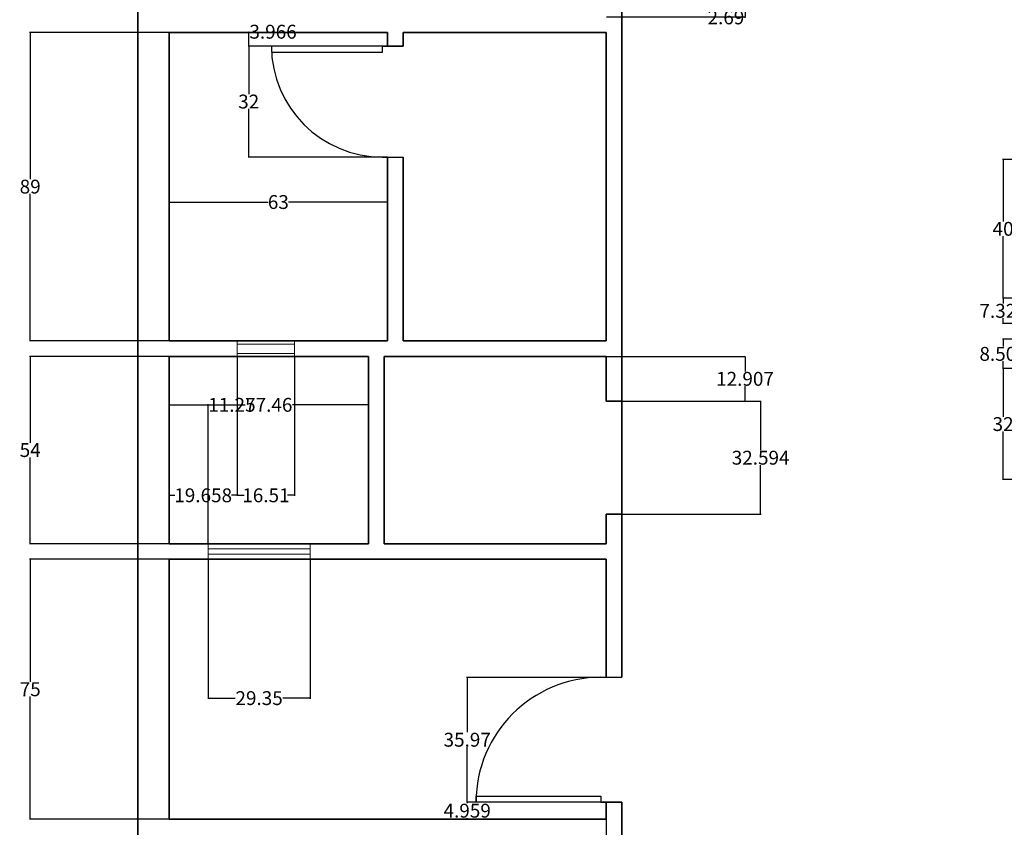
# Model space of a CAD drawing. Units: inches. Extents: x 1353 to 1853, y 16593 to 17433.
# Tile 2 of 4: x 1355 to 1639, y 16947 to 17180. Entities that reach past the tile are written whole.
import ezdxf

# ---------------------------------------------------------------- set-up
doc = ezdxf.new("R2010")
doc.units = ezdxf.units.IN
doc.header["$MEASUREMENT"] = 0
for name, color, linetype, lineweight in [('A-ANNO-DIMS', 2, 'Continuous', 18), ('A-DOOR', 3, 'Continuous', 25), ('A-GLAZ', 4, 'Continuous', 18), ('A-WALL', 7, 'Continuous', 35)]:
    doc.layers.add(name, color=color, linetype=linetype, lineweight=lineweight)
doc.styles.get("Standard").update_dxf_attribs({"font": 'arial.ttf'})
doc.dimstyles.get("Standard").update_dxf_attribs({"dimtxt": 4, "dimasz": 0.18, "dimexe": 0.18, "dimexo": 0.0625, "dimgap": 0.09, "dimtad": 0, "dimtih": 1, "dimtoh": 1, "dimdec": 0, "dimzin": 0, "dimdsep": 46, "dimlunit": 3, "dimtxsty": 'Standard', "dimcen": 0.09, "dimadec": 0, "dimazin": 0, "dimtfac": 1, "dimtdec": 0, "dimtofl": 0, "dimtmove": 0, "dimatfit": 3, "dimfxl": 1, "dimtolj": 1, "dimtzin": 0, "dimarcsym": 0})

# ---------------------------------------------------------------- blocks, each defined once
blk = doc.blocks.new('*U3')
for p, q in [((0, 0), (0, -6)), ((36, 0), (36, -6))]:
    blk.add_line(p, q)
blk.add_lwpolyline([(0, 0), (0, 36), (1.75, 36), (1.75, 0)], close=True)
blk.add_arc((0, 0), 36, 0, 90)
blk = doc.blocks.new('*U8')
for p, q in [((0, 0), (0, -6)), ((-32, 0), (-32, -6))]:
    blk.add_line(p, q)
blk.add_lwpolyline([(0, 0), (0, 32), (-1.75, 32), (-1.75, 0)], close=True)
blk.add_arc((0, 0), 32, 90, 180)
blk = doc.blocks.new('*D17')
at = {"layer": 'A-ANNO-DIMS', "color": 0, "lineweight": -2, "transparency": 16777216}
for p, q in [((1397.82, 17176.28), (1357.65, 17176.28)), ((1357.83, 17176.1), (1357.83, 17133.91)), ((1357.83, 17087.46), (1357.83, 17129.65)), ((1397.82, 17087.28), (1357.65, 17087.28))]:
    blk.add_line(p, q, dxfattribs=at)
at = {"layer": 'A-ANNO-DIMS', "color": 0, "transparency": 16777216}
for points in [[(1357.8, 17176.1), (1357.86, 17176.1), (1357.83, 17176.28)], [(1357.8, 17087.46), (1357.86, 17087.46), (1357.83, 17087.28)]]:
    blk.add_solid(points, dxfattribs=at)
at = {"layer": 'Defpoints', "color": 0, "transparency": 16777216}
for p in [(1357.83, 17176.28), (1397.88, 17176.28), (1397.88, 17087.28)]:
    blk.add_point(p, dxfattribs=at)
at = {"layer": 'A-ANNO-DIMS', "color": 0, "transparency": 16777216, "insert": (1357.83, 17131.78), "char_height": 4, "attachment_point": 5}
blk.add_mtext('\\A1;89', dxfattribs=at)
blk = doc.blocks.new('*D18')
at = {"layer": 'A-ANNO-DIMS', "color": 0, "lineweight": -2, "transparency": 16777216}
for p, q in [((1397.82, 17082.78), (1357.65, 17082.78)), ((1357.83, 17082.6), (1357.83, 17057.9)), ((1357.83, 17028.96), (1357.83, 17053.66)), ((1397.82, 17028.78), (1357.65, 17028.78))]:
    blk.add_line(p, q, dxfattribs=at)
at = {"layer": 'A-ANNO-DIMS', "color": 0, "transparency": 16777216}
for points in [[(1357.8, 17082.6), (1357.86, 17082.6), (1357.83, 17082.78)], [(1357.8, 17028.96), (1357.86, 17028.96), (1357.83, 17028.78)]]:
    blk.add_solid(points, dxfattribs=at)
at = {"layer": 'Defpoints', "color": 0, "transparency": 16777216}
for p in [(1357.83, 17082.78), (1397.88, 17082.78), (1397.88, 17028.78)]:
    blk.add_point(p, dxfattribs=at)
at = {"layer": 'A-ANNO-DIMS', "color": 0, "transparency": 16777216, "insert": (1357.83, 17055.78), "char_height": 4, "attachment_point": 5}
blk.add_mtext('\\A1;54', dxfattribs=at)
blk = doc.blocks.new('*D19')
at = {"layer": 'A-ANNO-DIMS', "color": 0, "lineweight": -2, "transparency": 16777216}
for p, q in [((1397.82, 17024.28), (1357.65, 17024.28)), ((1357.83, 17024.1), (1357.83, 16988.9)), ((1357.83, 16949.46), (1357.83, 16984.66)), ((1397.82, 16949.28), (1357.65, 16949.28))]:
    blk.add_line(p, q, dxfattribs=at)
at = {"layer": 'A-ANNO-DIMS', "color": 0, "transparency": 16777216}
for points in [[(1357.8, 17024.1), (1357.86, 17024.1), (1357.83, 17024.28)], [(1357.8, 16949.46), (1357.86, 16949.46), (1357.83, 16949.28)]]:
    blk.add_solid(points, dxfattribs=at)
at = {"layer": 'Defpoints', "color": 0, "transparency": 16777216}
for p in [(1357.83, 17024.28), (1397.88, 17024.28), (1397.88, 16949.28)]:
    blk.add_point(p, dxfattribs=at)
at = {"layer": 'A-ANNO-DIMS', "color": 0, "transparency": 16777216, "insert": (1357.83, 16986.78), "char_height": 4, "attachment_point": 5}
blk.add_mtext('\\A1;75', dxfattribs=at)
blk = doc.blocks.new('*D30')
at = {"layer": 'A-ANNO-DIMS', "color": 0, "lineweight": -2, "transparency": 16777216}
for p, q in [((1397.88, 17087.34), (1397.88, 17127.51)), ((1398.06, 17127.33), (1426.42, 17127.33)), ((1460.7, 17127.33), (1432.35, 17127.33)), ((1460.88, 17087.34), (1460.88, 17127.51))]:
    blk.add_line(p, q, dxfattribs=at)
at = {"layer": 'A-ANNO-DIMS', "color": 0, "transparency": 16777216}
for points in [[(1398.06, 17127.36), (1398.06, 17127.3), (1397.88, 17127.33)], [(1460.7, 17127.36), (1460.7, 17127.3), (1460.88, 17127.33)]]:
    blk.add_solid(points, dxfattribs=at)
at = {"layer": 'Defpoints', "color": 0, "transparency": 16777216}
for p in [(1460.88, 17127.33), (1397.88, 17087.28), (1460.88, 17087.28)]:
    blk.add_point(p, dxfattribs=at)
at = {"layer": 'A-ANNO-DIMS', "color": 0, "transparency": 16777216, "insert": (1429.38, 17127.33), "char_height": 4, "attachment_point": 5}
blk.add_mtext('\\A1;63', dxfattribs=at)
blk = doc.blocks.new('*D31')
at = {"layer": 'A-ANNO-DIMS', "color": 0, "lineweight": -2, "transparency": 16777216}
for p, q in [((1397.88, 17028.84), (1397.88, 17069.01)), ((1398.06, 17068.83), (1419.78, 17068.83)), ((1455.17, 17068.83), (1433.45, 17068.83)), ((1455.35, 17028.84), (1455.35, 17069.01))]:
    blk.add_line(p, q, dxfattribs=at)
at = {"layer": 'A-ANNO-DIMS', "color": 0, "transparency": 16777216}
for points in [[(1398.06, 17068.86), (1398.06, 17068.8), (1397.88, 17068.83)], [(1455.17, 17068.86), (1455.17, 17068.8), (1455.35, 17068.83)]]:
    blk.add_solid(points, dxfattribs=at)
at = {"layer": 'Defpoints', "color": 0, "transparency": 16777216}
for p in [(1455.35, 17068.83), (1397.88, 17028.78), (1455.35, 17028.78)]:
    blk.add_point(p, dxfattribs=at)
at = {"layer": 'A-ANNO-DIMS', "color": 0, "transparency": 16777216, "insert": (1426.62, 17068.83), "char_height": 4, "attachment_point": 5}
blk.add_mtext('\\A1;57.46', dxfattribs=at)
blk = doc.blocks.new('*D33')
at = {"layer": 'A-ANNO-DIMS', "color": 0, "lineweight": -2, "transparency": 16777216}
for p, q in [((1523.88, 16954.18), (1523.88, 16914.01)), ((1528.38, 16954.18), (1528.38, 16914.01)), ((1523.88, 16914.19), (1523.7, 16914.19)), ((1528.2, 16914.19), (1524.06, 16914.19))]:
    blk.add_line(p, q, dxfattribs=at)
at = {"layer": 'A-ANNO-DIMS', "color": 0, "transparency": 16777216}
for points in [[(1524.06, 16914.22), (1524.06, 16914.16), (1523.88, 16914.19)], [(1528.2, 16914.22), (1528.2, 16914.16), (1528.38, 16914.19)]]:
    blk.add_solid(points, dxfattribs=at)
at = {"layer": 'Defpoints', "color": 0, "transparency": 16777216}
for p in [(1523.88, 16954.24), (1528.38, 16954.24), (1523.88, 16914.19)]:
    blk.add_point(p, dxfattribs=at)
at = {"layer": 'A-ANNO-DIMS', "color": 0, "transparency": 16777216, "insert": (1519.88, 16914.19), "char_height": 4, "attachment_point": 5}
blk.add_mtext('\\A1;4.5', dxfattribs=at)
blk = doc.blocks.new('*D56')
at = {"layer": 'A-ANNO-DIMS', "color": 0, "lineweight": -2, "transparency": 16777216}
for p, q in [((1523.95, 17183.47), (1564.11, 17183.47)), ((1563.93, 17183.29), (1563.93, 17180.96)), ((1523.95, 17180.78), (1564.11, 17180.78)), ((1563.93, 17180.6), (1563.75, 17180.6)), ((1563.93, 17180.78), (1563.93, 17180.6))]:
    blk.add_line(p, q, dxfattribs=at)
at = {"layer": 'A-ANNO-DIMS', "color": 0, "transparency": 16777216}
for points in [[(1563.9, 17183.29), (1563.96, 17183.29), (1563.93, 17183.47)], [(1563.9, 17180.96), (1563.96, 17180.96), (1563.93, 17180.78)]]:
    blk.add_solid(points, dxfattribs=at)
at = {"layer": 'Defpoints', "color": 0, "transparency": 16777216}
for p in [(1523.88, 17183.47), (1523.88, 17180.78), (1563.93, 17180.78)]:
    blk.add_point(p, dxfattribs=at)
at = {"layer": 'A-ANNO-DIMS', "color": 0, "transparency": 16777216, "insert": (1558.43, 17180.6), "char_height": 4, "attachment_point": 5}
blk.add_mtext('\\A1;2.69', dxfattribs=at)
blk = doc.blocks.new('*D57')
at = {"layer": 'A-ANNO-DIMS', "color": 0, "lineweight": -2, "transparency": 16777216}
for p, q in [((1460.82, 17172.32), (1420.65, 17172.32)), ((1420.83, 17172.14), (1420.83, 17158.45)), ((1420.83, 17140.5), (1420.83, 17154.18)), ((1460.82, 17140.32), (1420.65, 17140.32))]:
    blk.add_line(p, q, dxfattribs=at)
at = {"layer": 'A-ANNO-DIMS', "color": 0, "transparency": 16777216}
for points in [[(1420.8, 17172.14), (1420.86, 17172.14), (1420.83, 17172.32)], [(1420.8, 17140.5), (1420.86, 17140.5), (1420.83, 17140.32)]]:
    blk.add_solid(points, dxfattribs=at)
at = {"layer": 'Defpoints', "color": 0, "transparency": 16777216}
for p in [(1420.83, 17172.32), (1460.88, 17172.32), (1460.88, 17140.32)]:
    blk.add_point(p, dxfattribs=at)
at = {"layer": 'A-ANNO-DIMS', "color": 0, "transparency": 16777216, "insert": (1420.83, 17156.32), "char_height": 4, "attachment_point": 5}
blk.add_mtext('\\A1;32', dxfattribs=at)
blk = doc.blocks.new('*D58')
at = {"layer": 'A-ANNO-DIMS', "color": 0, "lineweight": -2, "transparency": 16777216}
for p, q in [((1460.82, 17176.28), (1420.65, 17176.28)), ((1420.83, 17176.28), (1420.83, 17176.46)), ((1420.83, 17176.46), (1421.01, 17176.46)), ((1420.83, 17172.5), (1420.83, 17176.1)), ((1460.82, 17172.32), (1420.65, 17172.32))]:
    blk.add_line(p, q, dxfattribs=at)
at = {"layer": 'A-ANNO-DIMS', "color": 0, "transparency": 16777216}
for points in [[(1420.8, 17176.1), (1420.86, 17176.1), (1420.83, 17176.28)], [(1420.8, 17172.5), (1420.86, 17172.5), (1420.83, 17172.32)]]:
    blk.add_solid(points, dxfattribs=at)
at = {"layer": 'Defpoints', "color": 0, "transparency": 16777216}
for p in [(1420.83, 17176.28), (1460.88, 17176.28), (1460.88, 17172.32)]:
    blk.add_point(p, dxfattribs=at)
at = {"layer": 'A-ANNO-DIMS', "color": 0, "transparency": 16777216, "insert": (1427.85, 17176.46), "char_height": 4, "attachment_point": 5}
blk.add_mtext('\\A1;3.966', dxfattribs=at)
blk = doc.blocks.new('*D59')
at = {"layer": 'A-ANNO-DIMS', "color": 0, "lineweight": -2, "transparency": 16777216}
for p, q in [((1523.82, 16990.21), (1483.65, 16990.21)), ((1483.83, 16990.03), (1483.83, 16974.36)), ((1483.83, 16954.42), (1483.83, 16970.09)), ((1523.82, 16954.24), (1483.65, 16954.24))]:
    blk.add_line(p, q, dxfattribs=at)
at = {"layer": 'A-ANNO-DIMS', "color": 0, "transparency": 16777216}
for points in [[(1483.8, 16990.03), (1483.86, 16990.03), (1483.83, 16990.21)], [(1483.8, 16954.42), (1483.86, 16954.42), (1483.83, 16954.24)]]:
    blk.add_solid(points, dxfattribs=at)
at = {"layer": 'Defpoints', "color": 0, "transparency": 16777216}
for p in [(1483.83, 16990.21), (1523.88, 16990.21), (1523.88, 16954.24)]:
    blk.add_point(p, dxfattribs=at)
at = {"layer": 'A-ANNO-DIMS', "color": 0, "transparency": 16777216, "insert": (1483.83, 16972.22), "char_height": 4, "attachment_point": 5}
blk.add_mtext('\\A1;35.97', dxfattribs=at)
blk = doc.blocks.new('*D61')
at = {"layer": 'A-ANNO-DIMS', "color": 0, "lineweight": -2, "transparency": 16777216}
for p, q in [((1678.32, 17139.6), (1638.15, 17139.6)), ((1638.33, 17139.42), (1638.33, 17121.73)), ((1638.33, 17099.78), (1638.33, 17117.47)), ((1678.32, 17099.6), (1638.15, 17099.6))]:
    blk.add_line(p, q, dxfattribs=at)
at = {"layer": 'A-ANNO-DIMS', "color": 0, "transparency": 16777216}
for points in [[(1638.3, 17139.42), (1638.36, 17139.42), (1638.33, 17139.6)], [(1638.3, 17099.78), (1638.36, 17099.78), (1638.33, 17099.6)]]:
    blk.add_solid(points, dxfattribs=at)
at = {"layer": 'Defpoints', "color": 0, "transparency": 16777216}
for p in [(1638.33, 17139.6), (1678.38, 17139.6), (1678.38, 17099.6)]:
    blk.add_point(p, dxfattribs=at)
at = {"layer": 'A-ANNO-DIMS', "color": 0, "transparency": 16777216, "insert": (1638.33, 17119.6), "char_height": 4, "attachment_point": 5}
blk.add_mtext('\\A1;40', dxfattribs=at)
blk = doc.blocks.new('*D62')
at = {"layer": 'A-ANNO-DIMS', "color": 0, "lineweight": -2, "transparency": 16777216}
for p, q in [((1678.32, 17079.28), (1638.15, 17079.28)), ((1638.33, 17079.1), (1638.33, 17065.41)), ((1638.33, 17047.46), (1638.33, 17061.14)), ((1678.32, 17047.28), (1638.15, 17047.28))]:
    blk.add_line(p, q, dxfattribs=at)
at = {"layer": 'A-ANNO-DIMS', "color": 0, "transparency": 16777216}
for points in [[(1638.3, 17079.1), (1638.36, 17079.1), (1638.33, 17079.28)], [(1638.3, 17047.46), (1638.36, 17047.46), (1638.33, 17047.28)]]:
    blk.add_solid(points, dxfattribs=at)
at = {"layer": 'Defpoints', "color": 0, "transparency": 16777216}
for p in [(1638.33, 17079.28), (1678.38, 17079.28), (1678.38, 17047.28)]:
    blk.add_point(p, dxfattribs=at)
at = {"layer": 'A-ANNO-DIMS', "color": 0, "transparency": 16777216, "insert": (1638.33, 17063.28), "char_height": 4, "attachment_point": 5}
blk.add_mtext('\\A1;32', dxfattribs=at)
blk = doc.blocks.new('*D68')
at = {"layer": 'A-ANNO-DIMS', "color": 0, "lineweight": -2, "transparency": 16777216}
for p, q in [((1397.88, 17082.72), (1397.88, 17042.55)), ((1417.54, 17082.72), (1417.54, 17042.55)), ((1398.06, 17042.73), (1399.5, 17042.73)), ((1417.36, 17042.73), (1415.92, 17042.73))]:
    blk.add_line(p, q, dxfattribs=at)
at = {"layer": 'A-ANNO-DIMS', "color": 0, "transparency": 16777216}
for points in [[(1398.06, 17042.76), (1398.06, 17042.7), (1397.88, 17042.73)], [(1417.36, 17042.76), (1417.36, 17042.7), (1417.54, 17042.73)]]:
    blk.add_solid(points, dxfattribs=at)
at = {"layer": 'Defpoints', "color": 0, "transparency": 16777216}
for p in [(1397.88, 17082.78), (1417.54, 17082.78), (1397.88, 17042.73)]:
    blk.add_point(p, dxfattribs=at)
at = {"layer": 'A-ANNO-DIMS', "color": 0, "transparency": 16777216, "insert": (1407.71, 17042.73), "char_height": 4, "attachment_point": 5}
blk.add_mtext('\\A1;19.658', dxfattribs=at)
blk = doc.blocks.new('*D69')
at = {"layer": 'A-ANNO-DIMS', "color": 0, "lineweight": -2, "transparency": 16777216}
for p, q in [((1417.54, 17082.72), (1417.54, 17042.55)), ((1434.05, 17082.72), (1434.05, 17042.55)), ((1417.72, 17042.73), (1419.53, 17042.73)), ((1433.87, 17042.73), (1432.06, 17042.73))]:
    blk.add_line(p, q, dxfattribs=at)
at = {"layer": 'A-ANNO-DIMS', "color": 0, "transparency": 16777216}
for points in [[(1417.72, 17042.76), (1417.72, 17042.7), (1417.54, 17042.73)], [(1433.87, 17042.76), (1433.87, 17042.7), (1434.05, 17042.73)]]:
    blk.add_solid(points, dxfattribs=at)
at = {"layer": 'Defpoints', "color": 0, "transparency": 16777216}
for p in [(1417.54, 17082.78), (1434.05, 17082.78), (1417.54, 17042.73)]:
    blk.add_point(p, dxfattribs=at)
at = {"layer": 'A-ANNO-DIMS', "color": 0, "transparency": 16777216, "insert": (1425.8, 17042.73), "char_height": 4, "attachment_point": 5}
blk.add_mtext('\\A1;16.51', dxfattribs=at)
blk = doc.blocks.new('*D70')
at = {"layer": 'A-ANNO-DIMS', "color": 0, "lineweight": -2, "transparency": 16777216}
for p, q in [((1397.88, 17028.84), (1397.88, 17069.01)), ((1398.06, 17068.83), (1408.97, 17068.83)), ((1409.15, 17028.84), (1409.15, 17069.01)), ((1409.15, 17068.83), (1409.33, 17068.83))]:
    blk.add_line(p, q, dxfattribs=at)
at = {"layer": 'A-ANNO-DIMS', "color": 0, "transparency": 16777216}
for points in [[(1398.06, 17068.86), (1398.06, 17068.8), (1397.88, 17068.83)], [(1408.97, 17068.86), (1408.97, 17068.8), (1409.15, 17068.83)]]:
    blk.add_solid(points, dxfattribs=at)
at = {"layer": 'Defpoints', "color": 0, "transparency": 16777216}
for p in [(1409.15, 17068.83), (1397.88, 17028.78), (1409.15, 17028.78)]:
    blk.add_point(p, dxfattribs=at)
at = {"layer": 'A-ANNO-DIMS', "color": 0, "transparency": 16777216, "insert": (1415.99, 17068.83), "char_height": 4, "attachment_point": 5}
blk.add_mtext('\\A1;11.27', dxfattribs=at)
blk = doc.blocks.new('*D71')
at = {"layer": 'A-ANNO-DIMS', "color": 0, "lineweight": -2, "transparency": 16777216}
for p, q in [((1409.15, 17024.22), (1409.15, 16984.05)), ((1438.51, 17024.22), (1438.51, 16984.05)), ((1409.33, 16984.23), (1416.94, 16984.23)), ((1438.33, 16984.23), (1430.72, 16984.23))]:
    blk.add_line(p, q, dxfattribs=at)
at = {"layer": 'A-ANNO-DIMS', "color": 0, "transparency": 16777216}
for points in [[(1409.33, 16984.26), (1409.33, 16984.2), (1409.15, 16984.23)], [(1438.33, 16984.26), (1438.33, 16984.2), (1438.51, 16984.23)]]:
    blk.add_solid(points, dxfattribs=at)
at = {"layer": 'Defpoints', "color": 0, "transparency": 16777216}
for p in [(1409.15, 17024.28), (1438.51, 17024.28), (1409.15, 16984.23)]:
    blk.add_point(p, dxfattribs=at)
at = {"layer": 'A-ANNO-DIMS', "color": 0, "transparency": 16777216, "insert": (1423.83, 16984.23), "char_height": 4, "attachment_point": 5}
blk.add_mtext('\\A1;29.35', dxfattribs=at)
blk = doc.blocks.new('*D72')
at = {"layer": 'A-ANNO-DIMS', "color": 0, "lineweight": -2, "transparency": 16777216}
for p, q in [((1528.45, 17069.87), (1568.61, 17069.87)), ((1568.43, 17069.69), (1568.43, 17055.71)), ((1568.43, 17037.46), (1568.43, 17051.44)), ((1528.45, 17037.28), (1568.61, 17037.28))]:
    blk.add_line(p, q, dxfattribs=at)
at = {"layer": 'A-ANNO-DIMS', "color": 0, "transparency": 16777216}
for points in [[(1568.4, 17069.69), (1568.46, 17069.69), (1568.43, 17069.87)], [(1568.4, 17037.46), (1568.46, 17037.46), (1568.43, 17037.28)]]:
    blk.add_solid(points, dxfattribs=at)
at = {"layer": 'Defpoints', "color": 0, "transparency": 16777216}
for p in [(1528.38, 17069.87), (1528.38, 17037.28), (1568.43, 17037.28)]:
    blk.add_point(p, dxfattribs=at)
at = {"layer": 'A-ANNO-DIMS', "color": 0, "transparency": 16777216, "insert": (1568.43, 17053.58), "char_height": 4, "attachment_point": 5}
blk.add_mtext('\\A1;32.594', dxfattribs=at)
blk = doc.blocks.new('*D73')
at = {"layer": 'A-ANNO-DIMS', "color": 0, "lineweight": -2, "transparency": 16777216}
for p, q in [((1523.95, 17082.78), (1564.11, 17082.78)), ((1563.93, 17082.6), (1563.93, 17078.46)), ((1563.93, 17070.05), (1563.93, 17074.2)), ((1523.95, 17069.87), (1564.11, 17069.87))]:
    blk.add_line(p, q, dxfattribs=at)
at = {"layer": 'A-ANNO-DIMS', "color": 0, "transparency": 16777216}
for points in [[(1563.9, 17082.6), (1563.96, 17082.6), (1563.93, 17082.78)], [(1563.9, 17070.05), (1563.96, 17070.05), (1563.93, 17069.87)]]:
    blk.add_solid(points, dxfattribs=at)
at = {"layer": 'Defpoints', "color": 0, "transparency": 16777216}
for p in [(1523.88, 17082.78), (1523.88, 17069.87), (1563.93, 17069.87)]:
    blk.add_point(p, dxfattribs=at)
at = {"layer": 'A-ANNO-DIMS', "color": 0, "transparency": 16777216, "insert": (1563.93, 17076.33), "char_height": 4, "attachment_point": 5}
blk.add_mtext('\\A1;12.907', dxfattribs=at)
blk = doc.blocks.new('*D74')
at = {"layer": 'A-ANNO-DIMS', "color": 0, "lineweight": -2, "transparency": 16777216}
for p, q in [((1678.32, 17087.78), (1638.15, 17087.78)), ((1638.33, 17087.6), (1638.33, 17085.66)), ((1638.33, 17079.46), (1638.33, 17081.4)), ((1678.32, 17079.28), (1638.15, 17079.28))]:
    blk.add_line(p, q, dxfattribs=at)
at = {"layer": 'A-ANNO-DIMS', "color": 0, "transparency": 16777216}
for points in [[(1638.3, 17087.6), (1638.36, 17087.6), (1638.33, 17087.78)], [(1638.3, 17079.46), (1638.36, 17079.46), (1638.33, 17079.28)]]:
    blk.add_solid(points, dxfattribs=at)
at = {"layer": 'Defpoints', "color": 0, "transparency": 16777216}
for p in [(1638.33, 17087.78), (1678.38, 17087.78), (1678.38, 17079.28)]:
    blk.add_point(p, dxfattribs=at)
at = {"layer": 'A-ANNO-DIMS', "color": 0, "transparency": 16777216, "insert": (1638.33, 17083.53), "char_height": 4, "attachment_point": 5}
blk.add_mtext('\\A1;8.504', dxfattribs=at)
blk = doc.blocks.new('*D75')
at = {"layer": 'A-ANNO-DIMS', "color": 0, "lineweight": -2, "transparency": 16777216}
for p, q in [((1678.32, 17099.6), (1638.15, 17099.6)), ((1638.33, 17099.42), (1638.33, 17098.08)), ((1638.33, 17092.46), (1638.33, 17093.81)), ((1678.32, 17092.28), (1638.15, 17092.28))]:
    blk.add_line(p, q, dxfattribs=at)
at = {"layer": 'A-ANNO-DIMS', "color": 0, "transparency": 16777216}
for points in [[(1638.3, 17099.42), (1638.36, 17099.42), (1638.33, 17099.6)], [(1638.3, 17092.46), (1638.36, 17092.46), (1638.33, 17092.28)]]:
    blk.add_solid(points, dxfattribs=at)
at = {"layer": 'Defpoints', "color": 0, "transparency": 16777216}
for p in [(1638.33, 17099.6), (1678.38, 17099.6), (1678.38, 17092.28)]:
    blk.add_point(p, dxfattribs=at)
at = {"layer": 'A-ANNO-DIMS', "color": 0, "transparency": 16777216, "insert": (1638.33, 17095.94), "char_height": 4, "attachment_point": 5}
blk.add_mtext('\\A1;7.321', dxfattribs=at)
blk = doc.blocks.new('*D76')
at = {"layer": 'A-ANNO-DIMS', "color": 0, "lineweight": -2, "transparency": 16777216}
for p, q in [((1523.82, 16954.24), (1483.65, 16954.24)), ((1483.83, 16954.06), (1483.83, 16953.89)), ((1523.82, 16949.28), (1483.65, 16949.28)), ((1483.83, 16949.46), (1483.83, 16949.63))]:
    blk.add_line(p, q, dxfattribs=at)
at = {"layer": 'A-ANNO-DIMS', "color": 0, "transparency": 16777216}
for points in [[(1483.8, 16954.06), (1483.86, 16954.06), (1483.83, 16954.24)], [(1483.8, 16949.46), (1483.86, 16949.46), (1483.83, 16949.28)]]:
    blk.add_solid(points, dxfattribs=at)
at = {"layer": 'Defpoints', "color": 0, "transparency": 16777216}
for p in [(1483.83, 16954.24), (1523.88, 16954.24), (1523.88, 16949.28)]:
    blk.add_point(p, dxfattribs=at)
at = {"layer": 'A-ANNO-DIMS', "color": 0, "transparency": 16777216, "insert": (1483.83, 16951.76), "char_height": 4, "attachment_point": 5}
blk.add_mtext('\\A1;4.959', dxfattribs=at)

msp = doc.modelspace()

# ---------------------------------------------------------------- linework, layer by layer
at = {"layer": 'A-GLAZ'}
for p, q in [((1417.5423, 17082.7809), (1417.5423, 17087.2809)), ((1417.5423, 17087.2809), (1434.0526, 17087.2809)), ((1434.0526, 17087.2809), (1434.0526, 17082.7809)), ((1434.0526, 17086.3524), (1417.5423, 17086.3524)), ((1417.5423, 17082.7809), (1417.5423, 17084.555)), ((1417.5423, 17084.555), (1417.5423, 17083.6679)), ((1434.0526, 17083.6679), (1434.0526, 17086.3524)), ((1417.5423, 17083.6679), (1434.0526, 17083.6679)), ((1434.0526, 17082.7809), (1417.5423, 17082.7809)), ((1417.5423, 17082.7809), (1417.5423, 17082.7809)), ((1409.1544, 17024.2809), (1409.1544, 17028.7809)), ((1409.1544, 17028.7809), (1438.5066, 17028.7809)), ((1438.5066, 17027.2646), (1409.1544, 17027.2646)), ((1438.5066, 17028.7809), (1438.5066, 17024.2809)), ((1438.5066, 17025.1249), (1438.5066, 17027.2646)), ((1438.5066, 17025.7421), (1409.1544, 17025.7421)), ((1409.1544, 17024.2809), (1409.1544, 17025.1249)), ((1438.5066, 17024.2809), (1409.1544, 17024.2809)), ((1409.1544, 17024.2809), (1409.1544, 17024.2809)), ((1438.5066, 17025.1249), (1438.5066, 17025.7421))]:
    msp.add_line(p, q, dxfattribs=at)
at = {"layer": 'A-WALL'}
for p, q in [((1388.8844, 16635.7809), (1388.8844, 17432.7809)), ((1528.3844, 17176.2809), (1528.3844, 17183.4674)), ((1397.8844, 17176.2809), (1455.9979, 17176.2809)), ((1397.8844, 17087.2809), (1397.8844, 17176.2809)), ((1455.9979, 17176.2809), (1460.8844, 17176.2809)), ((1460.8844, 17172.3152), (1460.8844, 17176.2809)), ((1465.3844, 17176.2809), (1523.8844, 17176.2809)), ((1465.3844, 17172.3152), (1465.3844, 17176.2809)), ((1523.8844, 17176.2809), (1523.8844, 17168.5457)), ((1528.3844, 17176.2809), (1528.3844, 17168.5457)), ((1465.3844, 17172.3152), (1460.8844, 17172.3152)), ((1523.8844, 17133.8664), (1523.8844, 17168.5457)), ((1528.3844, 17133.8664), (1528.3844, 17168.5457)), ((1460.8844, 17087.2809), (1460.8844, 17140.3152)), ((1465.3844, 17087.2809), (1465.3844, 17140.3152)), ((1523.8844, 17133.8664), (1523.8844, 17087.2809)), ((1528.3844, 17133.8664), (1528.3844, 17082.7809)), ((1397.8844, 17087.2809), (1460.8844, 17087.2809)), ((1465.3844, 17087.2809), (1523.8844, 17087.2809)), ((1397.8844, 17082.7809), (1445.8844, 17082.7809)), ((1397.8844, 17028.7809), (1397.8844, 17082.7809)), ((1445.8844, 17082.7809), (1455.3459, 17082.7809)), ((1455.3459, 17028.7809), (1455.3459, 17082.7809)), ((1459.8459, 17028.7809), (1459.8459, 17082.7809)), ((1459.8459, 17082.7809), (1465.3844, 17082.7809)), ((1465.3844, 17082.7809), (1523.8844, 17082.7809)), ((1523.8844, 17082.7809), (1523.8844, 17069.8743)), ((1528.3844, 17082.7809), (1528.3844, 17069.8743)), ((1528.3844, 17069.8743), (1523.8844, 17069.8743)), ((1528.3844, 17037.2799), (1528.3844, 17069.8743)), ((1523.8844, 17037.2799), (1528.3844, 17037.2799)), ((1523.8844, 17037.2799), (1523.8844, 17028.7809)), ((1528.3844, 17037.2799), (1528.3844, 17024.2809)), ((1397.8844, 17028.7809), (1445.8844, 17028.7809)), ((1445.8844, 17028.7809), (1455.3459, 17028.7809)), ((1459.8459, 17028.7809), (1523.8844, 17028.7809)), ((1397.8844, 17024.2809), (1450.3844, 17024.2809)), ((1397.8844, 16949.2809), (1397.8844, 17024.2809)), ((1450.3844, 17024.2809), (1459.8459, 17024.2809)), ((1459.8459, 17024.2809), (1523.8844, 17024.2809)), ((1523.8844, 17024.2809), (1523.8844, 16990.2086)), ((1528.3844, 17024.2809), (1528.3844, 16990.2398)), ((1523.8844, 16949.2809), (1523.8844, 16954.2398)), ((1523.8844, 16954.2398), (1528.3844, 16954.2398)), ((1528.3844, 16944.7809), (1528.3844, 16954.2398)), ((1397.8844, 16949.2809), (1459.8459, 16949.2809)), ((1459.8459, 16949.2809), (1523.8844, 16949.2809))]:
    msp.add_line(p, q, dxfattribs=at)

# ---------------------------------------------------------------- block references
at = {"layer": 'A-DOOR', "rotation": 90}
for name, p in [('*U8', (1459.3844, 17172.3152)), ('*U3', (1522.3844, 16954.2398))]:
    msp.add_blockref(name, p, dxfattribs=at)

# ---------------------------------------------------------------- dimensions: what is measured, and where the dimension line sits
at = {"layer": 'A-ANNO-DIMS'}
for base, p1, p2, angle, override, picture, middle in [((1563.9344, 17180.7809), (1523.8844, 17183.4674), (1523.8844, 17180.7809), 270, {"dimdec": 2, "dimlfac": 1, "dimrnd": 0, "dimzin": 0, "dimdsep": 46, "dimlunit": 2}, '*D56', (1558.4311, 17180.6009)), ((1420.8344, 17176.2809), (1460.8844, 17172.3152), (1460.8844, 17176.2809), 90, {"dimdec": 3, "dimlfac": 1, "dimrnd": 0, "dimzin": 0, "dimdsep": 46, "dimlunit": 2}, '*D58', (1427.8506, 17176.4609)), ((1357.8344, 17176.2809), (1397.8844, 17087.2809), (1397.8844, 17176.2809), 90, {"dimdec": 0, "dimlfac": 1, "dimrnd": 0, "dimzin": 0, "dimdsep": 46, "dimlunit": 2}, '*D17', (1357.8344, 17131.7809)), ((1420.8344, 17172.3152), (1460.8844, 17140.3152), (1460.8844, 17172.3152), 90, {"dimdec": 0, "dimlfac": 1, "dimrnd": 0, "dimzin": 0, "dimdsep": 46, "dimlunit": 2}, '*D57', (1420.8344, 17156.3152)), ((1638.3344, 17139.6023), (1678.3844, 17099.6023), (1678.3844, 17139.6023), 90, {"dimdec": 0, "dimlfac": 1, "dimrnd": 0, "dimzin": 0, "dimdsep": 46, "dimlunit": 2}, '*D61', (1638.3344, 17119.6023)), ((1638.3344, 17099.6023), (1678.3844, 17092.2809), (1678.3844, 17099.6023), 90, {"dimdec": 3, "dimlfac": 1, "dimrnd": 0, "dimzin": 0, "dimdsep": 46, "dimlunit": 2}, '*D75', (1638.3344, 17095.9416)), ((1638.3344, 17087.7809), (1678.3844, 17079.277), (1678.3844, 17087.7809), 90, {"dimdec": 3, "dimlfac": 1, "dimrnd": 0, "dimzin": 0, "dimdsep": 46, "dimlunit": 2}, '*D74', (1638.3344, 17083.529)), ((1357.8344, 17082.7809), (1397.8844, 17028.7809), (1397.8844, 17082.7809), 90, {"dimdec": 0, "dimlfac": 1, "dimrnd": 0, "dimzin": 0, "dimdsep": 46, "dimlunit": 2}, '*D18', (1357.8344, 17055.7809)), ((1397.8844, 17042.7309), (1417.5423, 17082.7809), (1397.8844, 17082.7809), 180, {"dimdec": 3, "dimlfac": 1, "dimrnd": 0, "dimzin": 0, "dimdsep": 46, "dimlunit": 2}, '*D68', (1407.7133, 17042.7309)), ((1417.5423, 17042.7309), (1434.0526, 17082.7809), (1417.5423, 17082.7809), 180, {"dimdec": 2, "dimlfac": 1, "dimrnd": 0, "dimzin": 0, "dimdsep": 46, "dimlunit": 2}, '*D69', (1425.7974, 17042.7309)), ((1563.9344, 17069.8743), (1523.8844, 17082.7809), (1523.8844, 17069.8743), 270, {"dimdec": 3, "dimlfac": 1, "dimrnd": 0, "dimzin": 0, "dimdsep": 46, "dimlunit": 2}, '*D73', (1563.9344, 17076.3276)), ((1638.3344, 17079.277), (1678.3844, 17047.277), (1678.3844, 17079.277), 90, {"dimdec": 0, "dimlfac": 1, "dimrnd": 0, "dimzin": 0, "dimdsep": 46, "dimlunit": 2}, '*D62', (1638.3344, 17063.277)), ((1568.4344, 17037.2799), (1528.3844, 17069.8743), (1528.3844, 17037.2799), 270, {"dimdec": 3, "dimlfac": 1, "dimrnd": 0, "dimzin": 0, "dimdsep": 46, "dimlunit": 2}, '*D72', (1568.4344, 17053.5771)), ((1357.8344, 17024.2809), (1397.8844, 16949.2809), (1397.8844, 17024.2809), 90, {"dimdec": 0, "dimlfac": 1, "dimrnd": 0, "dimzin": 0, "dimdsep": 46, "dimlunit": 2}, '*D19', (1357.8344, 16986.7809)), ((1409.1544, 16984.2309), (1438.5066, 17024.2809), (1409.1544, 17024.2809), 180, {"dimdec": 2, "dimlfac": 1, "dimrnd": 0, "dimzin": 0, "dimdsep": 46, "dimlunit": 2}, '*D71', (1423.8305, 16984.2309)), ((1483.8344, 16990.2086), (1523.8844, 16954.2398), (1523.8844, 16990.2086), 90, {"dimdec": 2, "dimlfac": 1, "dimrnd": 0, "dimzin": 0, "dimdsep": 46, "dimlunit": 2}, '*D59', (1483.8344, 16972.2242)), ((1483.8344, 16954.2398), (1523.8844, 16949.2809), (1523.8844, 16954.2398), 90, {"dimdec": 3, "dimlfac": 1, "dimrnd": 0, "dimzin": 0, "dimdsep": 46, "dimlunit": 2}, '*D76', (1483.8344, 16951.7604)), ((1523.8844, 16914.1898), (1528.3844, 16954.2398), (1523.8844, 16954.2398), 180, {"dimdec": 1, "dimlfac": 1, "dimrnd": 0, "dimzin": 0, "dimdsep": 46, "dimlunit": 2}, '*D33', (1519.8777, 16914.1898))]:
    dim = msp.add_linear_dim(base=base, p1=p1, p2=p2, angle=angle, dimstyle='Standard', override=override, dxfattribs=at)
    dim.commit()
    dim.dimension.update_dxf_attribs({"geometry": picture, "text_midpoint": middle})
for base, p1, p2, override, picture, middle in [((1460.8844, 17127.3309), (1397.8844, 17087.2809), (1460.8844, 17087.2809), {"dimdec": 0, "dimlfac": 1, "dimrnd": 0, "dimzin": 0, "dimdsep": 46, "dimlunit": 2}, '*D30', (1429.3844, 17127.3309)), ((1455.3459, 17068.8309), (1397.8844, 17028.7809), (1455.3459, 17028.7809), {"dimdec": 2, "dimlfac": 1, "dimrnd": 0, "dimzin": 0, "dimdsep": 46, "dimlunit": 2}, '*D31', (1426.6151, 17068.8309)), ((1409.1544, 17068.8309), (1397.8844, 17028.7809), (1409.1544, 17028.7809), {"dimdec": 2, "dimlfac": 1, "dimrnd": 0, "dimzin": 0, "dimdsep": 46, "dimlunit": 2}, '*D70', (1415.9851, 17068.8309))]:
    dim = msp.add_linear_dim(base=base, p1=p1, p2=p2, dimstyle='Standard', override=override, dxfattribs=at)
    dim.commit()
    dim.dimension.update_dxf_attribs({"geometry": picture, "text_midpoint": middle})

doc.saveas('drawing.dxf')
